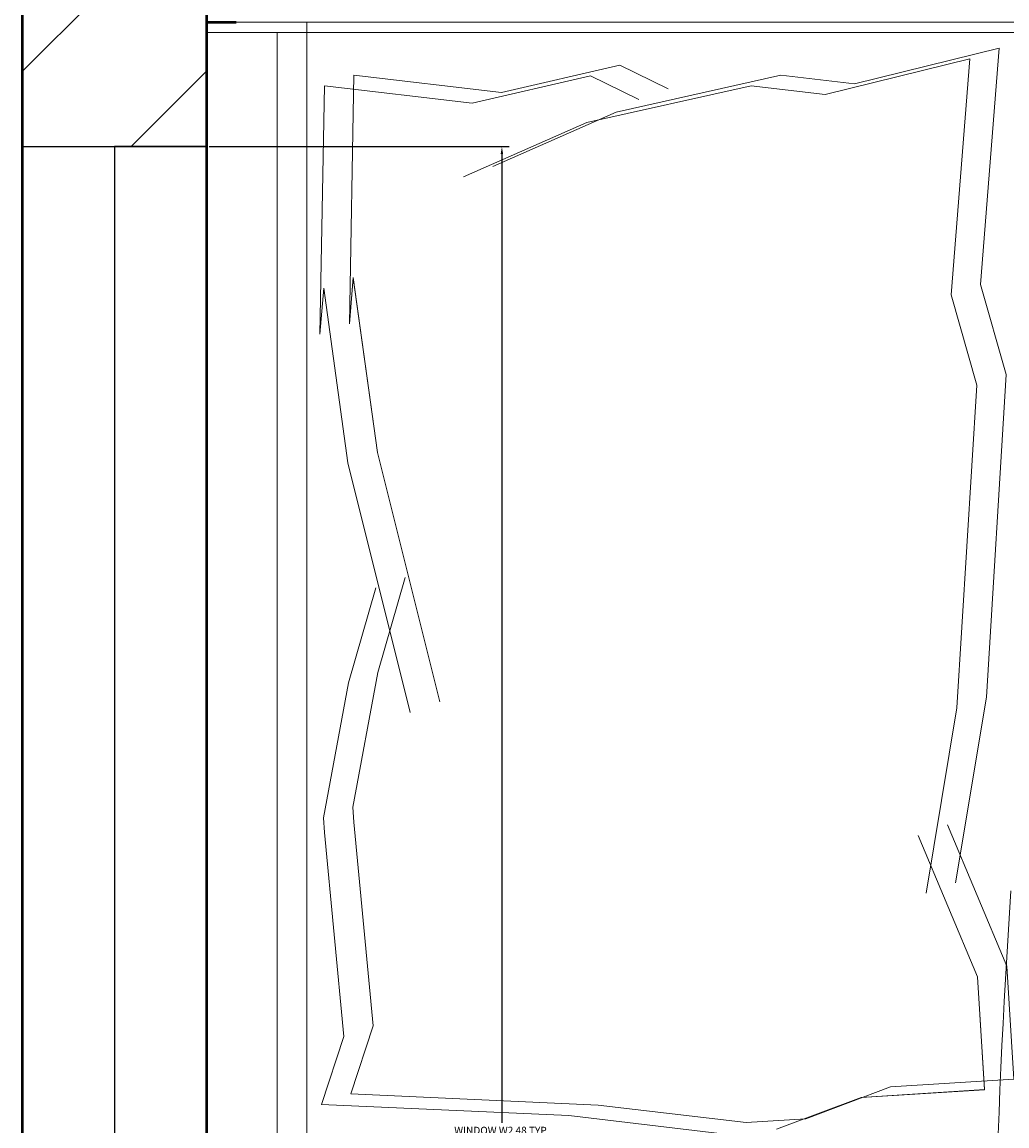
# Model space of a CAD drawing. Units: inches. Extents: x 1901 to 2863, y 888 to 2433.
# Tile 57 of 91: x 2025 to 2049, y 2161 to 2188. Entities that reach past the tile are written whole.
import ezdxf

# ---------------------------------------------------------------- set-up
doc = ezdxf.new("R2010")
doc.units = ezdxf.units.IN
for name, color, linetype, lineweight in [('A-ANNO-DIMS', 2, 'Continuous', 18), ('A-FURN', 8, 'Continuous', 18), ('A-GLAZ', 3, 'Continuous', 25), ('A-WALL', 7, 'Continuous', 50), ('A-WALL-PATT', 8, 'Continuous', 13)]:
    doc.layers.add(name, color=color, linetype=linetype, lineweight=lineweight)
doc.styles.get("Standard").update_dxf_attribs({"font": 'arial.ttf'})
doc.dimstyles.get("Standard").update_dxf_attribs({"dimtxt": 0.18, "dimasz": 0.18, "dimexe": 0.18, "dimexo": 0.0625, "dimgap": 0.09, "dimtad": 0, "dimtih": 1, "dimtoh": 1, "dimdec": 4, "dimzin": 0, "dimdsep": 46, "dimtxsty": 'Standard', "dimcen": 0.09, "dimadec": 0, "dimazin": 0, "dimtfac": 1, "dimtdec": 4, "dimtofl": 0, "dimtmove": 0, "dimatfit": 3, "dimfxl": 1, "dimtolj": 1, "dimtzin": 0, "dimarcsym": 0})

# ---------------------------------------------------------------- blocks, each defined once
blk = doc.blocks.new('BED-DOUBLE')
for p, q in [((0.026, 57.778), (0.026, 4.122)), ((0.744, 57.778), (30.62, 57.778)), ((19.351, 57.142), (15.827, 56.271)), ((19.351, 57.141), (15.827, 56.271)), ((18.898, 51.38), (19.351, 57.142)), ((18.898, 51.379), (19.351, 57.141)), ((18.633, 56.885), (15.109, 56.014)), ((18.633, 56.885), (15.109, 56.014)), ((18.18, 51.123), (18.633, 56.885)), ((18.18, 51.123), (18.633, 56.885)), ((7.22, 56.058), (10.106, 56.726)), ((7.22, 56.058), (10.106, 56.726)), ((10.106, 56.726), (11.28, 56.149)), ((10.106, 56.726), (11.28, 56.149)), ((3.615, 56.483), (3.506, 50.417)), ((3.615, 56.483), (3.506, 50.418)), ((3.615, 56.483), (7.22, 56.058)), ((3.615, 56.483), (7.22, 56.058)), ((6.502, 55.801), (9.388, 56.47)), ((6.502, 55.802), (9.388, 56.47)), ((9.388, 56.47), (10.563, 55.893)), ((9.388, 56.47), (10.563, 55.893)), ((14.025, 56.483), (10.015, 55.582)), ((14.025, 56.483), (10.015, 55.582)), ((15.827, 56.271), (14.025, 56.483)), ((15.827, 56.271), (14.025, 56.483)), ((2.897, 56.227), (2.788, 50.161)), ((2.897, 56.227), (2.788, 50.161)), ((2.897, 56.227), (6.502, 55.801)), ((2.897, 56.227), (6.502, 55.802)), ((13.307, 56.227), (9.297, 55.326)), ((13.307, 56.227), (9.297, 55.326)), ((15.109, 56.014), (13.307, 56.227)), ((15.109, 56.014), (13.307, 56.227)), ((10.015, 55.582), (7.007, 54.256)), ((10.015, 55.582), (7.007, 54.256)), ((9.297, 55.326), (6.289, 53.999)), ((9.297, 55.326), (6.289, 54)), ((3.506, 50.418), (3.598, 51.544)), ((3.506, 50.417), (3.598, 51.543)), ((3.598, 51.544), (4.19, 47.279)), ((3.598, 51.543), (4.19, 47.279)), ((2.788, 50.161), (2.881, 51.287)), ((2.788, 50.161), (2.881, 51.287)), ((2.881, 51.287), (3.472, 47.023)), ((2.881, 51.287), (3.472, 47.023)), ((19.523, 49.179), (18.898, 51.38)), ((19.523, 49.179), (18.898, 51.379)), ((18.806, 48.922), (18.18, 51.123)), ((18.806, 48.922), (18.18, 51.123)), ((19.039, 41.308), (19.523, 49.179)), ((19.039, 41.308), (19.523, 49.179)), ((18.322, 41.052), (18.806, 48.922)), ((18.322, 41.052), (18.806, 48.922)), ((4.19, 47.279), (5.709, 41.195)), ((4.19, 47.279), (5.709, 41.195)), ((3.472, 47.023), (4.991, 40.938)), ((3.472, 47.023), (4.991, 40.938)), ((4.869, 44.232), (4.2, 41.913)), ((4.869, 44.232), (4.2, 41.914)), ((4.151, 43.976), (3.482, 41.657)), ((4.151, 43.975), (3.482, 41.657)), ((4.2, 41.914), (3.593, 38.623)), ((4.2, 41.913), (3.593, 38.623)), ((3.482, 41.657), (2.875, 38.367)), ((3.482, 41.657), (2.875, 38.367)), ((18.291, 36.782), (19.039, 41.308)), ((18.291, 36.781), (19.039, 41.308)), ((17.573, 36.525), (18.322, 41.052)), ((17.573, 36.525), (18.322, 41.052)), ((3.593, 38.623), (3.615, 38.263)), ((3.593, 38.623), (3.615, 38.263)), ((2.875, 38.367), (2.897, 38.006)), ((2.875, 38.367), (2.897, 38.007)), ((3.615, 38.263), (4.088, 33.291)), ((3.615, 38.263), (4.088, 33.291)), ((2.897, 38.007), (3.371, 33.035)), ((2.897, 38.006), (3.371, 33.035)), ((19.538, 34.745), (18.096, 38.192)), ((19.538, 34.745), (18.096, 38.192)), ((18.82, 34.489), (17.378, 37.936)), ((18.82, 34.488), (17.378, 37.936)), ((19.71, 31.991), (19.538, 34.745)), ((19.71, 31.991), (19.538, 34.745)), ((18.993, 31.735), (18.82, 34.489)), ((18.993, 31.734), (18.82, 34.488)), ((4.088, 33.291), (3.542, 31.631)), ((4.088, 33.291), (3.542, 31.631)), ((3.371, 33.035), (2.824, 31.374)), ((3.371, 33.035), (2.824, 31.375)), ((14.64, 31.024), (16.706, 31.803)), ((14.64, 31.024), (16.706, 31.803)), ((16.706, 31.803), (19.71, 31.991)), ((16.706, 31.803), (19.71, 31.991)), ((3.542, 31.631), (9.577, 31.358)), ((3.542, 31.631), (9.577, 31.358)), ((13.922, 30.767), (15.988, 31.547)), ((13.922, 30.767), (15.988, 31.547)), ((15.988, 31.547), (18.993, 31.735)), ((15.988, 31.547), (18.993, 31.734)), ((2.824, 31.375), (8.859, 31.101)), ((2.824, 31.374), (8.859, 31.101)), ((9.577, 31.358), (13.182, 30.933)), ((9.577, 31.358), (13.182, 30.932)), ((8.859, 31.101), (12.464, 30.676)), ((8.859, 31.101), (12.464, 30.676)), ((13.182, 30.932), (14.64, 31.024)), ((13.182, 30.933), (14.64, 31.024))]:
    blk.add_line(p, q)
blk.add_arc((204.426, 23.944), 185.219, 176.08655, 186.78213)
blk.add_arc((204.426, 23.944), 185.219, 176.08655, 186.78213)
blk = doc.blocks.new('WIN-48')
for p, q in [((48, 4.5), (48, 0)), ((48, 2.25), (0, 2.25)), ((48, 0), (48, 2.25))]:
    blk.add_line(p, q)
blk = doc.blocks.new('*D21')
at = {"layer": 'A-ANNO-DIMS', "color": 0, "lineweight": -2, "transparency": 16777216}
for p, q in [((2029.489, 2184.739), (2036.806, 2184.739)), ((2036.626, 2184.559), (2036.626, 2160.923)), ((2036.626, 2136.919), (2036.626, 2160.556)), ((2029.489, 2136.739), (2036.806, 2136.739))]:
    blk.add_line(p, q, dxfattribs=at)
at = {"layer": 'A-ANNO-DIMS', "color": 0, "transparency": 16777216}
for points in [[(2036.596, 2184.559), (2036.656, 2184.559), (2036.626, 2184.739)], [(2036.596, 2136.919), (2036.656, 2136.919), (2036.626, 2136.739)]]:
    blk.add_solid(points, dxfattribs=at)
at = {"layer": 'Defpoints', "color": 0, "transparency": 16777216}
for p in [(2029.426, 2184.739), (2036.626, 2184.739), (2029.426, 2136.739)]:
    blk.add_point(p, dxfattribs=at)
at = {"layer": 'A-ANNO-DIMS', "color": 0, "transparency": 16777216, "insert": (2036.626, 2160.739), "char_height": 0.18, "attachment_point": 5}
blk.add_mtext('\\A1;WINDOW W2 48 TYP.', dxfattribs=at)
blk = doc.blocks.new('*D22')
at = {"layer": 'A-ANNO-DIMS', "color": 0, "lineweight": -2, "transparency": 16777216}
for p, q in [((2024.926, 2184.802), (2024.926, 2192.119)), ((2029.426, 2184.802), (2029.426, 2192.119)), ((2025.106, 2191.939), (2026.718, 2191.939)), ((2029.246, 2191.939), (2027.634, 2191.939))]:
    blk.add_line(p, q, dxfattribs=at)
at = {"layer": 'A-ANNO-DIMS', "color": 0, "transparency": 16777216}
for points in [[(2025.106, 2191.969), (2025.106, 2191.909), (2024.926, 2191.939)], [(2029.246, 2191.969), (2029.246, 2191.909), (2029.426, 2191.939)]]:
    blk.add_solid(points, dxfattribs=at)
at = {"layer": 'Defpoints', "color": 0, "transparency": 16777216}
for p in [(2024.926, 2191.939), (2024.926, 2184.739), (2029.426, 2184.739)]:
    blk.add_point(p, dxfattribs=at)
at = {"layer": 'A-ANNO-DIMS', "color": 0, "transparency": 16777216, "insert": (2027.176, 2191.939), "char_height": 0.18, "attachment_point": 5}
blk.add_mtext('\\A1;5 TYP.', dxfattribs=at)

msp = doc.modelspace()

# ---------------------------------------------------------------- hatches: boundary and pattern name
at = {"layer": 'A-WALL-PATT'}
h = msp.add_hatch(dxfattribs=at)
h.set_pattern_fill('ANSI32', color=256)
h.paths.add_polyline_path([(2192.501, 2274.134), (2141.264, 2274.134), (2141.264, 2269.634), (2192.501, 2269.634)])
h.paths.add_polyline_path([(2259.926, 2274.134), (2216.501, 2274.134), (2216.501, 2269.634), (2255.426, 2269.634), (2255.426, 2214.634), (2250.809, 2214.634), (2250.809, 2210.134), (2259.926, 2210.134), (2259.926, 2215.134), (2271.756, 2215.134), (2271.756, 2217.384), (2271.756, 2219.634), (2259.926, 2219.634)])
h.paths.add_polyline_path([(2171.426, 2269.634), (2166.926, 2269.634), (2166.926, 2219.634), (2121.238, 2219.634), (2121.238, 2215.134), (2166.926, 2215.134), (2166.926, 2083.134), (2161.807, 2083.134), (2161.807, 2078.634), (2171.426, 2078.634), (2176.996, 2078.634), (2176.996, 2080.884), (2176.996, 2083.134), (2171.426, 2083.134), (2171.426, 2210.134), (2230.912, 2210.134), (2230.912, 2212.384), (2230.912, 2214.634), (2171.426, 2214.634)])
h.paths.add_polyline_path([(2117.264, 2274.134), (2089.426, 2274.134), (2089.426, 2219.634), (2081.136, 2219.634), (2081.136, 2215.134), (2089.426, 2215.134), (2098.004, 2215.134), (2098.004, 2217.384), (2098.004, 2219.634), (2093.926, 2219.634), (2093.926, 2269.634), (2117.264, 2269.634), (2117.264, 2271.884)])
h.paths.add_polyline_path([(2343.426, 2219.634), (2329.295, 2219.634), (2329.295, 2215.134), (2338.926, 2215.134), (2338.926, 2184.739), (2343.426, 2184.739)])
h.paths.add_polyline_path([(2338.926, 2083.134), (2329.295, 2083.134), (2208.966, 2083.134), (2208.966, 2078.634), (2338.926, 2078.634)])
h.paths.add_polyline_path([(2343.426, 2136.739), (2338.926, 2136.739), (2338.926, 1872.634), (2343.426, 1872.634)])
h.paths.add_polyline_path([(2343.426, 1863.634), (2397.68, 1863.634), (2397.68, 1821.634), (2384.138, 1821.634), (2384.138, 1812.634), (2418.33, 1812.634), (2418.33, 1817.134), (2418.33, 1821.634), (2406.68, 1821.634), (2406.68, 1863.634), (2459.499, 1863.634), (2459.499, 1821.634), (2447.138, 1821.634), (2447.138, 1812.634), (2459.499, 1812.634), (2468.499, 1812.634), (2468.499, 1872.634), (2394.426, 1872.634), (2334.426, 1872.634), (2334.426, 1812.634), (2343.426, 1812.634), (2353.251, 1812.634), (2353.251, 1821.634), (2343.426, 1821.634)])
h.paths.add_polyline_path([(2510.014, 1872.634), (2468.499, 1872.634), (2468.499, 1868.134), (2510.014, 1868.134)])
h.paths.add_polyline_path([(2514.009, 1817.134), (2468.499, 1817.134), (2468.499, 1812.634), (2482.114, 1812.634), (2482.114, 1800.606), (2486.614, 1800.606), (2486.614, 1812.634), (2514.009, 1812.634)])
h.paths.add_polyline_path([(2299.247, 1814.884), (2299.247, 1817.134), (2295.926, 1817.134), (2295.926, 1854.169), (2293.676, 1854.169), (2291.426, 1854.169), (2291.426, 1817.134), (2266.109, 1817.134), (2266.109, 1812.634), (2299.247, 1812.634)])
h.paths.add_polyline_path([(2218.109, 1817.134), (2206.46, 1817.134), (2171.426, 1817.134), (2171.426, 1949.134), (2190.1, 1949.134), (2190.1, 1953.634), (2163.468, 1953.634), (2163.468, 1949.134), (2166.926, 1949.134), (2166.926, 1817.134), (2114.297, 1817.134), (2114.297, 1812.634), (2218.109, 1812.634)])
h.paths.add_polyline_path([(2029.426, 1970.922), (2024.926, 1970.922), (2024.926, 1912.717), (2029.426, 1912.717)])
h.paths.add_polyline_path([(2132.297, 1953.634), (2113.926, 1953.634), (2113.926, 1975.888), (2111.676, 1975.888), (2109.426, 1975.888), (2109.426, 1953.634), (2029.426, 1953.634), (2029.426, 1949.134), (2132.297, 1949.134)])
h.paths.add_polyline_path([(2029.426, 1853.606), (2029.31, 1853.606), (2029.31, 1853.606), (2029.426, 1853.606), (2029.426, 1864.717), (2024.926, 1864.717), (2024.926, 1812.634), (2066.297, 1812.634), (2066.297, 1814.884), (2066.297, 1817.134), (2029.426, 1817.134)])
h.paths.add_polyline_path([(2122.926, 2010.088), (2120.676, 2010.088), (2118.426, 2010.088), (2118.426, 2006.134), (2029.426, 2006.134), (2029.426, 2001.634), (2109.426, 2001.634), (2109.426, 1998.041), (2113.926, 1998.041), (2113.926, 2001.634), (2122.926, 2001.634)])
h.paths.add_polyline_path([(2029.426, 2031.376), (2024.926, 2031.376), (2024.926, 1994.922), (2027.176, 1994.922), (2029.426, 1994.922)])
h.paths.add_polyline_path([(2029.426, 2136.739), (2024.926, 2136.739), (2024.926, 2067.376), (2027.176, 2067.376), (2029.426, 2067.376)])
h.paths.add_polyline_path([(2125.618, 2083.134), (2029.426, 2083.134), (2029.426, 2078.634), (2118.426, 2078.634), (2118.426, 2030.715), (2122.926, 2030.715), (2122.926, 2078.634), (2125.618, 2078.634)])
h.paths.add_polyline_path([(2029.426, 2215.134), (2040.468, 2215.134), (2040.468, 2217.384), (2040.468, 2219.634), (2024.926, 2219.634), (2024.926, 2184.739), (2029.426, 2184.739), (2029.426, 2187.778)])
h.paths.add_polyline_path([(2686.426, 2274.134), (2659.284, 2274.134), (2659.284, 2269.634), (2681.926, 2269.634), (2681.926, 2219.634), (2676.816, 2219.634), (2676.816, 2215.134), (2681.926, 2215.134), (2697.011, 2215.134), (2697.011, 2217.384), (2697.011, 2219.634), (2686.426, 2219.634)])
h.paths.add_polyline_path([(2609.926, 2269.634), (2635.284, 2269.634), (2635.284, 2274.134), (2571.431, 2274.134), (2571.431, 2269.634), (2605.426, 2269.634), (2605.426, 2214.634), (2549.098, 2214.634), (2549.098, 2210.134), (2605.426, 2210.134), (2605.426, 2083.134), (2601.014, 2083.134), (2601.014, 2080.884), (2601.014, 2078.634), (2609.926, 2078.634), (2616.162, 2078.634), (2616.162, 2080.884), (2616.162, 2083.134), (2609.926, 2083.134), (2609.926, 2215.134), (2651.465, 2215.134), (2651.465, 2217.384), (2651.465, 2219.634), (2609.926, 2219.634)])
h.paths.add_polyline_path([(2521.426, 2269.634), (2547.431, 2269.634), (2547.431, 2271.884), (2547.431, 2274.134), (2516.926, 2274.134), (2516.926, 2219.634), (2506.41, 2219.634), (2506.41, 2215.134), (2516.926, 2215.134), (2516.926, 2210.134), (2525.402, 2210.134), (2525.402, 2212.384), (2525.402, 2214.634), (2521.426, 2214.634)])
h.paths.add_polyline_path([(2456.011, 2219.634), (2439.426, 2219.634), (2439.426, 2187.888), (2443.926, 2187.888), (2443.926, 2215.134), (2456.011, 2215.134)])
h.paths.add_polyline_path([(2752.926, 2219.634), (2739.485, 2219.634), (2739.485, 2215.134), (2748.426, 2215.134), (2748.426, 2187.888), (2752.926, 2187.888)])
h.paths.add_polyline_path([(2752.926, 2139.888), (2748.426, 2139.888), (2748.426, 2083.134), (2648.416, 2083.134), (2648.416, 2078.634), (2654.926, 2078.634), (2654.926, 2039.437), (2659.426, 2039.437), (2659.426, 2078.634), (2748.426, 2078.634), (2748.426, 2063.429), (2752.926, 2063.429)])
h.paths.add_polyline_path([(2752.926, 2010.634), (2659.426, 2010.634), (2659.426, 2015.652), (2654.926, 2015.652), (2654.926, 2010.634), (2605.426, 2010.634), (2605.426, 1920.967), (2609.926, 1920.967), (2609.926, 2006.134), (2748.426, 2006.134), (2748.426, 1982.466), (2752.926, 1982.466)])
h.paths.add_polyline_path([(2752.926, 2027.429), (2748.426, 2027.429), (2748.426, 2010.634), (2752.926, 2010.634)])
h.paths.add_polyline_path([(2748.426, 1886.134), (2609.926, 1886.134), (2609.926, 1889.719), (2605.426, 1889.719), (2605.426, 1861.262), (2609.926, 1861.262), (2609.926, 1881.634), (2748.426, 1881.634)])
h.paths.add_polyline_path([(2456.855, 2228.831), (2498.401, 2228.831), (2498.401, 2247.488), (2456.855, 2247.488)], flags=9)
h.paths.add_polyline_path([(2038.602, 2237.418), (2080.174, 2237.418), (2080.174, 2256.075), (2038.602, 2256.075)], flags=9)
h.paths.add_polyline_path([(2292.009, 1062.394), (2539.932, 1062.394), (2539.932, 1099.487), (2292.009, 1099.487)], flags=9)
h.paths.add_polyline_path([(2424.91, 1832.253), (2448.513, 1832.253), (2448.513, 1846.678), (2424.91, 1846.678)], flags=25)
h.paths.add_polyline_path([(2359.076, 1832.253), (2382.678, 1832.253), (2382.678, 1846.678), (2359.076, 1846.678)], flags=25)
h.paths.add_polyline_path([(2352.899, 1684.802), (2367.543, 1684.802), (2367.543, 1697.167), (2352.899, 1697.167)], flags=9)
h.paths.add_polyline_path([(2079.288, 1755.826), (2169.024, 1755.826), (2169.024, 1774.372), (2079.288, 1774.372)], flags=9)
h.paths.add_polyline_path([(2404.09, 1373.857), (2404.09, 1463.593), (2385.544, 1463.593), (2385.544, 1373.857)], flags=9)
h.paths.add_polyline_path([(2268.091, 2236.371), (2309.636, 2236.371), (2309.636, 2255.028), (2268.091, 2255.028)], flags=9)
h.paths.add_polyline_path([(2575.96, 1700.951), (2665.696, 1700.951), (2665.696, 1719.498), (2575.96, 1719.498)], flags=9)
h.paths.add_polyline_path([(2302.962, 1878.474), (2329.524, 1878.474), (2329.524, 1888.777), (2302.962, 1888.777)], flags=9)
h.paths.add_polyline_path([(2097.415, 2240.576), (2126.573, 2240.576), (2126.573, 2259.233), (2097.415, 2259.233)], flags=9)
h.paths.add_polyline_path([(2208.725, 2246.124), (2237.882, 2246.124), (2237.882, 2264.781), (2208.725, 2264.781)], flags=9)
h.paths.add_polyline_path([(2038.147, 1925.958), (2076.987, 1925.958), (2076.987, 1944.615), (2038.147, 1944.615)], flags=9)
h.paths.add_polyline_path([(2239.144, 1926.672), (2288.465, 1926.672), (2288.465, 1945.329), (2239.144, 1945.329)], flags=9)
h.paths.add_polyline_path([(2175.429, 2007.33), (2212.356, 2007.33), (2212.356, 2025.987), (2175.429, 2025.987)], flags=9)
h.paths.add_polyline_path([(2225.034, 2091.794), (2263.875, 2091.794), (2263.875, 2110.451), (2225.034, 2110.451)], flags=9)
h.paths.add_polyline_path([(2035.398, 2098.478), (2074.238, 2098.478), (2074.238, 2117.135), (2035.398, 2117.135)], flags=9)
h.paths.add_polyline_path([(2050.102, 2029.209), (2083.26, 2029.209), (2083.26, 2047.866), (2050.102, 2047.866)], flags=9)
h.paths.add_polyline_path([(2069.677, 1956.719), (2098.835, 1956.719), (2098.835, 1975.376), (2069.677, 1975.376)], flags=25)
h.paths.add_polyline_path([(2328.62, 1753.336), (2361.663, 1753.336), (2361.663, 1771.993), (2328.62, 1771.993)], flags=9)
h.paths.add_polyline_path([(2395.162, 2060.888), (2395.162, 2140.654), (2378.676, 2140.654), (2378.676, 2060.888)], flags=9)
h.paths.add_polyline_path([(2463.728, 2059.02), (2492.886, 2059.02), (2492.886, 2077.677), (2463.728, 2077.677)], flags=9)
h.paths.add_polyline_path([(2458.027, 2181.536), (2496.868, 2181.536), (2496.868, 2200.194), (2458.027, 2200.194)], flags=9)
h.paths.add_polyline_path([(2527.577, 2243.074), (2556.735, 2243.074), (2556.735, 2261.731), (2527.577, 2261.731)], flags=9)
h.paths.add_polyline_path([(2694.461, 2232.767), (2736.033, 2232.767), (2736.033, 2251.425), (2694.461, 2251.425)], flags=9)
h.paths.add_polyline_path([(2637.821, 2249.225), (2666.979, 2249.225), (2666.979, 2267.882), (2637.821, 2267.882)], flags=9)
h.paths.add_polyline_path([(2623.687, 2183.541), (2662.528, 2183.541), (2662.528, 2202.199), (2623.687, 2202.199)], flags=9)
h.paths.add_polyline_path([(2691.965, 2021.5), (2725.124, 2021.5), (2725.124, 2040.157), (2691.965, 2040.157)], flags=9)
h.paths.add_polyline_path([(2621.043, 1975.912), (2662.335, 1975.912), (2662.335, 1994.569), (2621.043, 1994.569)], flags=25)
h.paths.add_polyline_path([(2479.032, 1927.62), (2519.844, 1927.62), (2519.844, 1946.277), (2479.032, 1946.277)], flags=9)
h.paths.add_polyline_path([(2670.941, 1849.076), (2716.005, 1849.076), (2716.005, 1867.734), (2670.941, 1867.734)], flags=9)
h.paths.add_polyline_path([(2523.613, 1782.956), (2550.175, 1782.956), (2550.175, 1793.26), (2523.613, 1793.26)], flags=9)
h.paths.add_polyline_path([(2450.841, 1207.331), (2492.386, 1207.331), (2492.386, 1225.989), (2450.841, 1225.989)], flags=9)
h.paths.add_polyline_path([(2527.751, 1203.841), (2556.908, 1203.841), (2556.908, 1222.499), (2527.751, 1222.499)], flags=9)
h.paths.add_polyline_path([(2639.111, 1207.2), (2668.268, 1207.2), (2668.268, 1225.857), (2639.111, 1225.857)], flags=9)
h.paths.add_polyline_path([(2692.594, 1218.965), (2734.167, 1218.965), (2734.167, 1237.623), (2692.594, 1237.623)], flags=9)
h.paths.add_polyline_path([(2669.266, 1366.329), (2708.106, 1366.329), (2708.106, 1384.987), (2669.266, 1384.987)], flags=9)
h.paths.add_polyline_path([(2463.313, 1358.031), (2502.153, 1358.031), (2502.153, 1376.688), (2463.313, 1376.688)], flags=9)
h.paths.add_polyline_path([(2494.725, 1449.963), (2531.652, 1449.963), (2531.652, 1468.62), (2494.725, 1468.62)], flags=9)
h.paths.add_polyline_path([(2675.565, 1422.157), (2708.724, 1422.157), (2708.724, 1440.815), (2675.565, 1440.815)], flags=9)
h.paths.add_polyline_path([(2685.634, 1493.891), (2714.792, 1493.891), (2714.792, 1512.548), (2685.634, 1512.548)], flags=9)
h.paths.add_polyline_path([(2686.805, 1529.913), (2725.645, 1529.913), (2725.645, 1548.57), (2686.805, 1548.57)], flags=9)
h.paths.add_polyline_path([(2503.651, 1537.991), (2552.972, 1537.991), (2552.972, 1556.648), (2503.651, 1556.648)], flags=9)
h.paths.add_polyline_path([(2291.713, 1643.504), (2318.275, 1643.504), (2318.275, 1653.807), (2291.713, 1653.807)], flags=9)
h.paths.add_polyline_path([(2450.626, 1610.52), (2477.189, 1610.52), (2477.189, 1620.824), (2450.626, 1620.824)], flags=9)
h.paths.add_polyline_path([(2359.985, 1551.814), (2422.253, 1551.814), (2422.253, 1562.117), (2359.985, 1562.117)], flags=9)
h.paths.add_polyline_path([(2280.106, 1249.006), (2321.651, 1249.006), (2321.651, 1267.663), (2280.106, 1267.663)], flags=9)
h.paths.add_polyline_path([(2164.057, 1274.232), (2193.215, 1274.232), (2193.215, 1292.889), (2164.057, 1292.889)], flags=9)
h.paths.add_polyline_path([(2118.21, 1277.694), (2151.252, 1277.694), (2151.252, 1296.351), (2118.21, 1296.351)], flags=9)
h.paths.add_polyline_path([(2031.946, 1268.529), (2073.519, 1268.529), (2073.519, 1287.187), (2031.946, 1287.187)], flags=9)
h.paths.add_polyline_path([(2050.199, 1409.079), (2089.04, 1409.079), (2089.04, 1427.736), (2050.199, 1427.736)], flags=9)
h.paths.add_polyline_path([(2243.743, 1421.032), (2282.584, 1421.032), (2282.584, 1439.689), (2243.743, 1439.689)], flags=9)
h.paths.add_polyline_path([(2190.746, 1509.769), (2231.558, 1509.769), (2231.558, 1528.426), (2190.746, 1528.426)], flags=9)
h.paths.add_polyline_path([(2058.392, 1475.415), (2091.55, 1475.415), (2091.55, 1494.073), (2058.392, 1494.073)], flags=9)
h.paths.add_polyline_path([(2062.447, 1553.09), (2091.605, 1553.09), (2091.605, 1571.747), (2062.447, 1571.747)], flags=9)
h.paths.add_polyline_path([(2219.524, 1590.365), (2266.147, 1590.365), (2266.147, 1609.022), (2219.524, 1609.022)], flags=9)
h.paths.add_polyline_path([(2041.072, 1584.188), (2079.912, 1584.188), (2079.912, 1602.845), (2041.072, 1602.845)], flags=9)

# ---------------------------------------------------------------- linework, layer by layer
at = {"layer": 'A-FURN'}
for p, q in [((2031.866, 2134.122), (2031.866, 2187.778)), ((2031.866, 2134.121), (2031.866, 2187.778)), ((2029.426, 2187.522), (2059.302, 2187.522)), ((2029.426, 2187.522), (2059.302, 2187.522)), ((2031.148, 2133.865), (2031.148, 2187.522)), ((2031.148, 2133.865), (2031.148, 2187.522))]:
    msp.add_line(p, q, dxfattribs=at)
at = {"layer": 'A-WALL'}
for p, q in [((2024.926, 2219.634), (2024.926, 1812.634)), ((2029.426, 2215.134), (2029.426, 1817.134)), ((2029.426, 2187.778), (2030.144, 2187.778))]:
    msp.add_line(p, q, dxfattribs=at)

# ---------------------------------------------------------------- block references
at = {"layer": 'A-FURN'}
msp.add_blockref('BED-DOUBLE', (2029.4, 2130), dxfattribs=at)
at = {"layer": 'A-GLAZ', "rotation": 90.00000000000097}
msp.add_blockref('WIN-48', (2029.426, 2136.74), dxfattribs=at)

# ---------------------------------------------------------------- dimensions: what is measured, and where the dimension line sits
at = {"layer": 'A-ANNO-DIMS'}
for base, p1, p2, angle, text, picture, middle in [((2024.926174575, 2191.939408848), (2029.426174575, 2184.739408848), (2024.926174575, 2184.739408848), 180, '<> TYP.', '*D22', (2027.176174575, 2191.939408848)), ((2036.626, 2184.739), (2029.426, 2136.739), (2029.426, 2184.739), 90, 'WINDOW W2 <> TYP.', '*D21', (2036.626, 2160.739))]:
    dim = msp.add_linear_dim(base=base, p1=p1, p2=p2, angle=angle, text=text, dimstyle='Standard', override={"dimdec": 0, "dimlfac": 1, "dimrnd": 0, "dimzin": 0, "dimdsep": 46, "dimlunit": 2}, dxfattribs=at)
    dim.commit()
    dim.dimension.update_dxf_attribs({"geometry": picture, "text_midpoint": middle})

doc.saveas('drawing.dxf')
